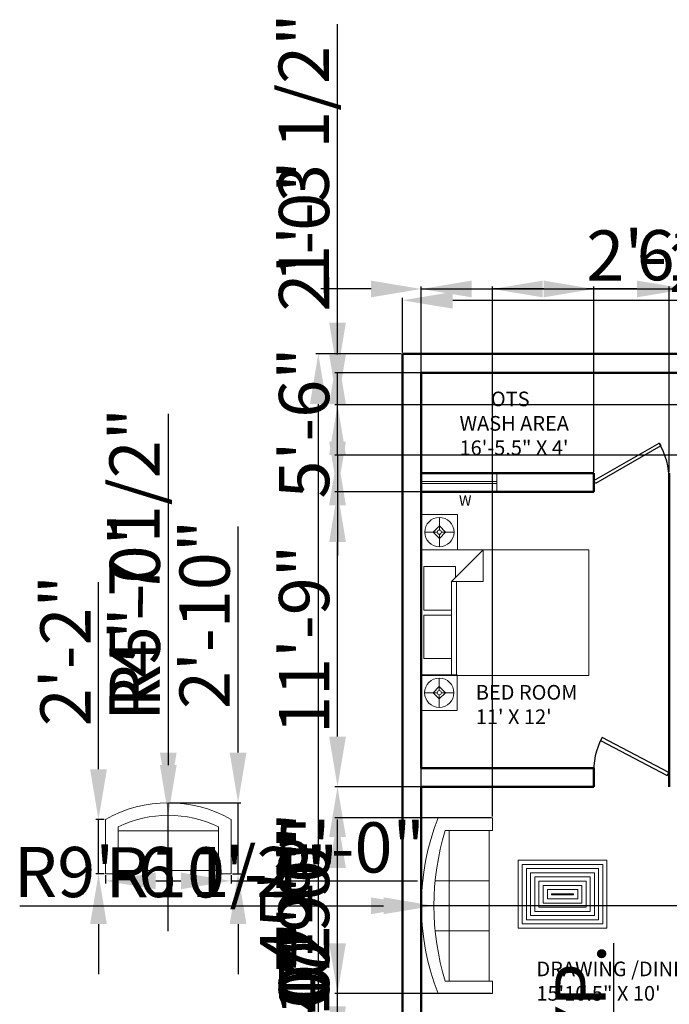
# Model space of a CAD drawing. Units: inches. Extents: x 1383 to 2465, y 1661 to 2415.
# Tile 2 of 4: x 1569 to 1880, y 1944 to 2415. Entities that reach past the tile are written whole.
import ezdxf

# ---------------------------------------------------------------- set-up
doc = ezdxf.new("R2010")
doc.units = ezdxf.units.IN
for name, color, linetype, lineweight in [('A-ANNO-DIMS', 2, 'Continuous', 18), ('A-ANNO-TEXT', 3, 'Continuous', 18), ('A-AREA-IDEN', 7, 'Continuous', 25), ('A-DOOR', 3, 'Continuous', 25), ('A-FURN', 8, 'Continuous', 18), ('A-GLAZ', 4, 'Continuous', 18), ('A-WALL', 7, 'Continuous', 50)]:
    doc.layers.add(name, color=color, linetype=linetype, lineweight=lineweight)
doc.styles.get("Standard").update_dxf_attribs({"font": 'arial.ttf'})
doc.dimstyles.new('ISO-25', dxfattribs={"dimtxt": 24, "dimasz": 24, "dimexe": 1.25, "dimexo": 0.625, "dimtad": 1, "dimdec": 0, "dimlunit": 3, "dimtxsty": 'Standard', "dimcen": 2.5, "dimadec": 0, "dimazin": 0, "dimtfac": 1, "dimtdec": 0, "dimtmove": 0, "dimatfit": 3, "dimfxl": 1, "dimarcsym": 0})

# ---------------------------------------------------------------- blocks, each defined once
blk = doc.blocks.new('*U4')
for p, q in [((0, 0), (0, -6)), ((-40, 0), (-40, -6))]:
    blk.add_line(p, q)
blk.add_lwpolyline([(0, 0), (-34.64, 20), (-35.52, 18.48), (-0.88, -1.52)], close=True)
blk.add_arc((0, 0), 40, 150, 180)
blk = doc.blocks.new('*U2')
for p, q in [((0, 0), (0, -6)), ((40, 0), (40, -6))]:
    blk.add_line(p, q)
blk.add_lwpolyline([(0, 0), (34.64, 20), (35.52, 18.48), (0.87, -1.52)], close=True)
blk.add_arc((0, 0), 40, 0, 30)
blk = doc.blocks.new('Bed - Queen')
for p, q in [((0, -80.00003), (0, 0)), ((0, 0), (59.99999, 0)), ((59.99999, 0), (59.99999, -80.00003)), ((7.99999, -1.2), (28.79998, -1.2)), ((7.99999, -14.4), (7.99999, -1.2)), ((28.79998, -1.2), (28.79998, -14.4)), ((31.19999, -1.2), (51.99999, -1.2)), ((31.19999, -14.4), (31.19999, -1.2)), ((51.99999, -1.2), (51.99999, -16.4)), ((0, -14.4), (44.8, -14.4)), ((44.8, -16.8), (0, -16.8)), ((59.99999, -29.6), (44.8, -14.4)), ((44.8, -14.4), (44.8, -29.6)), ((51.99999, -16.4), (46.79936, -16.4)), ((44.8, -29.6), (59.99999, -29.6)), ((59.99999, -80.00003), (0, -80.00003))]:
    blk.add_line(p, q)
blk = doc.blocks.new('Sofa - Roundback 7 ft.')
for p, q in [((-12.00002, -32.4421), (-12.00003, -6.5971)), ((11.99997, -32.4421), (11.99998, -6.5971)), ((-36.000027, -34), (-36.000027, -11.4696)), ((-35.999844, -13.3819), (35.9998, -13.3819)), ((35.99998, -34), (35.99998, -11.4696)), ((-36.000027, -32.4421), (35.99998, -32.4421))]:
    blk.add_line(p, q)
for points in [[(-36.000027, -34), (-42.000027, -34), (-42.000027, -8)], [(41.99998, -8), (41.99998, -34), (35.99998, -34)]]:
    blk.add_lwpolyline(points)
for centre, radius, start, end in [((0, -114.25), 114.25, 68.43141, 111.5686), ((-0.00001, -127.1968), 121.1968, 72.72033, 107.2797)]:
    blk.add_arc(centre, radius, start, end)
blk = doc.blocks.new('Sofa - Roundback Loveseat 5 ft.')
for p, q in [((0, -32.44198), (0, -5.99998)), ((-24, -33.99998), (-24, -11.46958)), ((-23.9998, -13.38178), (23.99986, -13.38178)), ((24.00004, -33.99998), (24.00004, -11.46958)), ((-24, -32.44198), (24.00004, -32.44198))]:
    blk.add_line(p, q)
for points in [[(-24, -33.99998), (-30, -33.99998), (-30, -7.99998)], [(30.00004, -7.99998), (30.00004, -33.99998), (24.00004, -33.99998)]]:
    blk.add_lwpolyline(points)
for centre, radius, start, end in [((0, -60.24998), 60.24998, 60.13715, 119.8628), ((0, -61.38438), 55.38444, 64.32083, 115.6792)]:
    blk.add_arc(centre, radius, start, end)
blk = doc.blocks.new('*D12')
at = {"layer": 'A-ANNO-DIMS', "color": 0, "lineweight": -2, "transparency": 16777216}
for p, q in [((1752.19, 2255.79), (1752.19, 2282.04)), ((1776.19, 2280.79), (2028.19, 2280.79)), ((2052.19, 2255.79), (2052.19, 2282.04))]:
    blk.add_line(p, q, dxfattribs=at)
at = {"layer": 'A-ANNO-DIMS', "color": 0, "transparency": 16777216}
for points in [[(1776.19, 2284.79), (1776.19, 2276.79), (1752.19, 2280.79)], [(2028.19, 2284.79), (2028.19, 2276.79), (2052.19, 2280.79)]]:
    blk.add_solid(points, dxfattribs=at)
at = {"layer": 'Defpoints', "color": 0, "transparency": 16777216}
for p in [(2052.19, 2280.79), (1752.19, 2255.16), (2052.19, 2255.16)]:
    blk.add_point(p, dxfattribs=at)
at = {"layer": 'A-ANNO-DIMS', "color": 0, "transparency": 16777216, "insert": (1902.19, 2293.67), "char_height": 24, "attachment_point": 5}
blk.add_mtext("25'", dxfattribs=at)
blk = doc.blocks.new('*D13')
at = {"layer": 'A-ANNO-DIMS', "color": 0, "lineweight": -2, "transparency": 16777216}
for p, q in [((1751.57, 2255.16), (1710.71, 2255.16)), ((1711.96, 2231.16), (1711.96, 1739.16)), ((1751.57, 1715.16), (1710.71, 1715.16))]:
    blk.add_line(p, q, dxfattribs=at)
at = {"layer": 'A-ANNO-DIMS', "color": 0, "transparency": 16777216}
for points in [[(1707.96, 2231.16), (1715.96, 2231.16), (1711.96, 2255.16)], [(1707.96, 1739.16), (1715.96, 1739.16), (1711.96, 1715.16)]]:
    blk.add_solid(points, dxfattribs=at)
at = {"layer": 'Defpoints', "color": 0, "transparency": 16777216}
for p in [(1752.19, 2255.16), (1711.96, 1715.16), (1752.19, 1715.16)]:
    blk.add_point(p, dxfattribs=at)
at = {"layer": 'A-ANNO-DIMS', "color": 0, "transparency": 16777216, "insert": (1699.13, 1985.16), "char_height": 24, "attachment_point": 5, "rotation": 90}
blk.add_mtext("45'", dxfattribs=at)
blk = doc.blocks.new('WIN-36IN')
for p, q in [((0, 36), (9, 36)), ((0, 0), (0, 36)), ((4, 0), (4, 36)), ((5, 36), (5, 0)), ((9, 36), (9, 0)), ((9, 0), (0, 0))]:
    blk.add_line(p, q)
blk = doc.blocks.new('Lamp - Table')
for p, q in [((0, 7), (0, 1)), ((-1, 0), (-7, 0)), ((0, 3), (-3, 0)), ((-3, 0), (0, -3)), ((3, 0), (0, 3)), ((0, -3), (3, 0)), ((1, 0), (7, 0)), ((0, -1), (0, -7))]:
    blk.add_line(p, q)
for radius in [7, 1]:
    blk.add_circle((0, 0), radius)
blk = doc.blocks.new('NIGHTSTAND-WITH-LAMP')
blk.add_lwpolyline([(0, 0), (17.23, 0), (17.23, 16.98), (0, 16.98)], close=True)
blk.add_blockref('Lamp - Table', (8.62, 8.49))
blk = doc.blocks.new('*D21')
at = {"layer": 'A-ANNO-DIMS', "color": 0, "lineweight": -2, "transparency": 16777216}
for p, q in [((1853.19, 1801.92), (1853.19, 1973.47)), ((1841.82, 1801.92), (1854.44, 1801.92)), ((1853.19, 1765.92), (1853.19, 1777.92)), ((1841.82, 1741.92), (1854.44, 1741.92))]:
    blk.add_line(p, q, dxfattribs=at)
at = {"layer": 'A-ANNO-DIMS', "color": 0, "transparency": 16777216}
for points in [[(1849.19, 1777.92), (1857.19, 1777.92), (1853.19, 1801.92)], [(1849.19, 1765.92), (1857.19, 1765.92), (1853.19, 1741.92)]]:
    blk.add_solid(points, dxfattribs=at)
at = {"layer": 'Defpoints', "color": 0, "transparency": 16777216}
for p in [(1841.19, 1801.92), (1853.19, 1801.92), (1841.19, 1741.92)]:
    blk.add_point(p, dxfattribs=at)
at = {"layer": 'A-ANNO-DIMS', "color": 0, "transparency": 16777216, "insert": (1840.32, 1899.7), "char_height": 24, "attachment_point": 5, "rotation": 90}
blk.add_mtext('5\'-0" TYP.', dxfattribs=at)
blk = doc.blocks.new('*D24')
at = {"layer": 'A-ANNO-DIMS', "color": 0, "lineweight": -2, "transparency": 16777216}
for p, q in [((1721.14, 1919.16), (1721.14, 2009.18)), ((1792.57, 1919.16), (1719.89, 1919.16)), ((1721.14, 1886.16), (1721.14, 1895.16)), ((1760.57, 1862.16), (1719.89, 1862.16))]:
    blk.add_line(p, q, dxfattribs=at)
at = {"layer": 'A-ANNO-DIMS', "color": 0, "transparency": 16777216}
for points in [[(1717.14, 1895.16), (1725.14, 1895.16), (1721.14, 1919.16)], [(1717.14, 1886.16), (1725.14, 1886.16), (1721.14, 1862.16)]]:
    blk.add_solid(points, dxfattribs=at)
at = {"layer": 'Defpoints', "color": 0, "transparency": 16777216}
for p in [(1721.14, 1919.16), (1793.19, 1919.16), (1761.19, 1862.16)]:
    blk.add_point(p, dxfattribs=at)
at = {"layer": 'A-ANNO-DIMS', "color": 0, "transparency": 16777216, "insert": (1708.26, 1976.17), "char_height": 24, "attachment_point": 5, "rotation": 90}
blk.add_mtext('4\'-9"', dxfattribs=at)
blk = doc.blocks.new('*D25')
at = {"layer": 'A-ANNO-DIMS', "color": 0, "lineweight": -2, "transparency": 16777216}
for p, q in [((1760.57, 2048.16), (1719.89, 2048.16)), ((1721.14, 1943.16), (1721.14, 2024.16)), ((1792.57, 1919.16), (1719.89, 1919.16))]:
    blk.add_line(p, q, dxfattribs=at)
at = {"layer": 'A-ANNO-DIMS', "color": 0, "transparency": 16777216}
for points in [[(1717.14, 2024.16), (1725.14, 2024.16), (1721.14, 2048.16)], [(1717.14, 1943.16), (1725.14, 1943.16), (1721.14, 1919.16)]]:
    blk.add_solid(points, dxfattribs=at)
at = {"layer": 'Defpoints', "color": 0, "transparency": 16777216}
for p in [(1721.14, 2048.16), (1761.19, 2048.16), (1793.19, 1919.16)]:
    blk.add_point(p, dxfattribs=at)
at = {"layer": 'A-ANNO-DIMS', "color": 0, "transparency": 16777216, "insert": (1708.26, 1983.66), "char_height": 24, "attachment_point": 5, "rotation": 90}
blk.add_mtext('10\'-9"', dxfattribs=at)
blk = doc.blocks.new('*D26')
at = {"layer": 'A-ANNO-DIMS', "color": 0, "lineweight": -2, "transparency": 16777216}
for p, q in [((1760.57, 2189.16), (1719.89, 2189.16)), ((1721.14, 2072.16), (1721.14, 2165.16)), ((1760.57, 2048.16), (1719.89, 2048.16))]:
    blk.add_line(p, q, dxfattribs=at)
at = {"layer": 'A-ANNO-DIMS', "color": 0, "transparency": 16777216}
for points in [[(1717.14, 2165.16), (1725.14, 2165.16), (1721.14, 2189.16)], [(1717.14, 2072.16), (1725.14, 2072.16), (1721.14, 2048.16)]]:
    blk.add_solid(points, dxfattribs=at)
at = {"layer": 'Defpoints', "color": 0, "transparency": 16777216}
for p in [(1721.14, 2189.16), (1761.19, 2189.16), (1761.19, 2048.16)]:
    blk.add_point(p, dxfattribs=at)
at = {"layer": 'A-ANNO-DIMS', "color": 0, "transparency": 16777216, "insert": (1708.26, 2118.66), "char_height": 24, "attachment_point": 5, "rotation": 90}
blk.add_mtext('11\'-9"', dxfattribs=at)
blk = doc.blocks.new('*D27')
at = {"layer": 'A-ANNO-DIMS', "color": 0, "lineweight": -2, "transparency": 16777216}
for p, q in [((1751.57, 2255.16), (1719.89, 2255.16)), ((1721.14, 2213.16), (1721.14, 2231.16)), ((1760.57, 2189.16), (1719.89, 2189.16))]:
    blk.add_line(p, q, dxfattribs=at)
at = {"layer": 'A-ANNO-DIMS', "color": 0, "transparency": 16777216}
for points in [[(1717.14, 2231.16), (1725.14, 2231.16), (1721.14, 2255.16)], [(1717.14, 2213.16), (1725.14, 2213.16), (1721.14, 2189.16)]]:
    blk.add_solid(points, dxfattribs=at)
at = {"layer": 'Defpoints', "color": 0, "transparency": 16777216}
for p in [(1721.14, 2255.16), (1752.19, 2255.16), (1761.19, 2189.16)]:
    blk.add_point(p, dxfattribs=at)
at = {"layer": 'A-ANNO-DIMS', "color": 0, "transparency": 16777216, "insert": (1708.26, 2222.16), "char_height": 24, "attachment_point": 5, "rotation": 90}
blk.add_mtext('5\'-6"', dxfattribs=at)
blk = doc.blocks.new('*D28')
at = {"layer": 'A-ANNO-DIMS', "color": 0, "lineweight": -2, "transparency": 16777216}
for p, q in [((1606.91, 2056.55), (1606.91, 2146.01)), ((1609.63, 2032.55), (1605.66, 2032.55)), ((1606.91, 2006.55), (1606.91, 2032.55)), ((1609.63, 2006.55), (1605.66, 2006.55)), ((1606.91, 1982.55), (1606.91, 1958.55))]:
    blk.add_line(p, q, dxfattribs=at)
at = {"layer": 'A-ANNO-DIMS', "color": 0, "transparency": 16777216}
for points in [[(1602.91, 2056.55), (1610.91, 2056.55), (1606.91, 2032.55)], [(1602.91, 1982.55), (1610.91, 1982.55), (1606.91, 2006.55)]]:
    blk.add_solid(points, dxfattribs=at)
at = {"layer": 'Defpoints', "color": 0, "transparency": 16777216}
for p in [(1606.91, 2032.55), (1610.26, 2032.55), (1610.26, 2006.55)]:
    blk.add_point(p, dxfattribs=at)
at = {"layer": 'A-ANNO-DIMS', "color": 0, "transparency": 16777216, "insert": (1594.23, 2113.28), "char_height": 24, "attachment_point": 5, "rotation": 90}
blk.add_mtext('2\'-2"', dxfattribs=at)
blk = doc.blocks.new('*D29')
at = {"layer": 'A-ANNO-DIMS', "color": 0, "lineweight": -2, "transparency": 16777216}
for p, q in [((1610.26, 2005.92), (1610.26, 2001.95)), ((1670.26, 2005.92), (1670.26, 2001.95)), ((1634.26, 2003.2), (1646.26, 2003.2)), ((1670.26, 2003.2), (1759.31, 2003.2))]:
    blk.add_line(p, q, dxfattribs=at)
at = {"layer": 'A-ANNO-DIMS', "color": 0, "transparency": 16777216}
for points in [[(1634.26, 2007.2), (1634.26, 1999.2), (1610.26, 2003.2)], [(1646.26, 2007.2), (1646.26, 1999.2), (1670.26, 2003.2)]]:
    blk.add_solid(points, dxfattribs=at)
at = {"layer": 'Defpoints', "color": 0, "transparency": 16777216}
for p in [(1610.26, 2006.55), (1670.26, 2006.55), (1670.26, 2003.2)]:
    blk.add_point(p, dxfattribs=at)
at = {"layer": 'A-ANNO-DIMS', "color": 0, "transparency": 16777216, "insert": (1726.78, 2016.08), "char_height": 24, "attachment_point": 5}
blk.add_mtext('5\'-0"', dxfattribs=at)
blk = doc.blocks.new('*D30')
at = {"layer": 'A-ANNO-DIMS', "color": 0, "lineweight": -2, "transparency": 16777216}
for p, q in [((1673.61, 2064.55), (1673.61, 2172.65)), ((1640.88, 2040.55), (1674.86, 2040.55)), ((1673.61, 2006.55), (1673.61, 2040.55)), ((1670.88, 2006.55), (1674.86, 2006.55)), ((1673.61, 1982.55), (1673.61, 1958.55))]:
    blk.add_line(p, q, dxfattribs=at)
at = {"layer": 'A-ANNO-DIMS', "color": 0, "transparency": 16777216}
for points in [[(1669.61, 2064.55), (1677.61, 2064.55), (1673.61, 2040.55)], [(1669.61, 1982.55), (1677.61, 1982.55), (1673.61, 2006.55)]]:
    blk.add_solid(points, dxfattribs=at)
at = {"layer": 'Defpoints', "color": 0, "transparency": 16777216}
for p in [(1640.26, 2040.55), (1673.61, 2040.55), (1670.26, 2006.55)]:
    blk.add_point(p, dxfattribs=at)
at = {"layer": 'A-ANNO-DIMS', "color": 0, "transparency": 16777216, "insert": (1660.73, 2130.6), "char_height": 24, "attachment_point": 5, "rotation": 90}
blk.add_mtext('2\'-10"', dxfattribs=at)
blk = doc.blocks.new('*D34')
at = {"layer": 'A-ANNO-DIMS', "color": 0, "lineweight": -2, "transparency": 16777216}
for p, q in [((1721.14, 2254.82), (1721.14, 2344.28)), ((2042.57, 2230.82), (1719.89, 2230.82)), ((1721.14, 2206.82), (1721.14, 2230.82)), ((2042.57, 2206.82), (1719.89, 2206.82)), ((1721.14, 2182.82), (1721.14, 2158.82))]:
    blk.add_line(p, q, dxfattribs=at)
at = {"layer": 'A-ANNO-DIMS', "color": 0, "transparency": 16777216}
for points in [[(1717.14, 2254.82), (1725.14, 2254.82), (1721.14, 2230.82)], [(1717.14, 2182.82), (1725.14, 2182.82), (1721.14, 2206.82)]]:
    blk.add_solid(points, dxfattribs=at)
at = {"layer": 'Defpoints', "color": 0, "transparency": 16777216}
for p in [(1721.14, 2230.82), (2043.19, 2230.82), (2043.19, 2206.82)]:
    blk.add_point(p, dxfattribs=at)
at = {"layer": 'A-ANNO-DIMS', "color": 0, "transparency": 16777216, "insert": (1708.26, 2311.55), "char_height": 24, "attachment_point": 5, "rotation": 90}
blk.add_mtext('2\'-0"', dxfattribs=at)
blk = doc.blocks.new('*D35')
at = {"layer": 'A-ANNO-DIMS', "color": 0, "lineweight": -2, "transparency": 16777216}
for p, q in [((1721.14, 2270.16), (1721.14, 2412.87)), ((2042.57, 2246.16), (1719.89, 2246.16)), ((1721.14, 2230.82), (1721.14, 2246.16)), ((2042.57, 2230.82), (1719.89, 2230.82)), ((1721.14, 2206.82), (1721.14, 2182.82))]:
    blk.add_line(p, q, dxfattribs=at)
at = {"layer": 'A-ANNO-DIMS', "color": 0, "transparency": 16777216}
for points in [[(1717.14, 2270.16), (1725.14, 2270.16), (1721.14, 2246.16)], [(1717.14, 2206.82), (1725.14, 2206.82), (1721.14, 2230.82)]]:
    blk.add_solid(points, dxfattribs=at)
at = {"layer": 'Defpoints', "color": 0, "transparency": 16777216}
for p in [(1721.14, 2246.16), (2043.19, 2246.16), (2043.19, 2230.82)]:
    blk.add_point(p, dxfattribs=at)
at = {"layer": 'A-ANNO-DIMS', "color": 0, "transparency": 16777216, "insert": (1708.1, 2353.52), "char_height": 24, "attachment_point": 5, "rotation": 90}
blk.add_mtext('1\'-3 1/2"', dxfattribs=at)
blk = doc.blocks.new('*D38')
at = {"layer": 'A-ANNO-DIMS', "color": 0, "lineweight": -2, "transparency": 16777216}
for p, q in [((1761.19, 2198.79), (1761.19, 2287.46)), ((1785.19, 2286.21), (1819.69, 2286.21)), ((1843.69, 2198.79), (1843.69, 2287.46)), ((1843.69, 2286.21), (2007.44, 2286.21))]:
    blk.add_line(p, q, dxfattribs=at)
at = {"layer": 'A-ANNO-DIMS', "color": 0, "transparency": 16777216}
for points in [[(1785.19, 2290.21), (1785.19, 2282.21), (1761.19, 2286.21)], [(1819.69, 2290.21), (1819.69, 2282.21), (1843.69, 2286.21)]]:
    blk.add_solid(points, dxfattribs=at)
at = {"layer": 'Defpoints', "color": 0, "transparency": 16777216}
for p in [(1843.69, 2286.21), (1761.19, 2198.16), (1843.69, 2198.16)]:
    blk.add_point(p, dxfattribs=at)
at = {"layer": 'A-ANNO-DIMS', "color": 0, "transparency": 16777216, "insert": (1937.57, 2299.25), "char_height": 24, "attachment_point": 5}
blk.add_mtext('6\'-10 1/2"', dxfattribs=at)
blk = doc.blocks.new('*D39')
at = {"layer": 'A-ANNO-DIMS', "color": 0, "lineweight": -2, "transparency": 16777216}
for p, q in [((1819.69, 2286.21), (1795.69, 2286.21)), ((1843.69, 2198.79), (1843.69, 2287.46)), ((1843.69, 2286.21), (1879.69, 2286.21)), ((1879.69, 2198.79), (1879.69, 2287.46)), ((1903.69, 2286.21), (1992.73, 2286.21))]:
    blk.add_line(p, q, dxfattribs=at)
at = {"layer": 'A-ANNO-DIMS', "color": 0, "transparency": 16777216}
for points in [[(1819.69, 2290.21), (1819.69, 2282.21), (1843.69, 2286.21)], [(1903.69, 2290.21), (1903.69, 2282.21), (1879.69, 2286.21)]]:
    blk.add_solid(points, dxfattribs=at)
at = {"layer": 'Defpoints', "color": 0, "transparency": 16777216}
for p in [(1879.69, 2286.21), (1843.69, 2198.16), (1879.69, 2198.16)]:
    blk.add_point(p, dxfattribs=at)
at = {"layer": 'A-ANNO-DIMS', "color": 0, "transparency": 16777216, "insert": (1960.21, 2299.1), "char_height": 24, "attachment_point": 5}
blk.add_mtext('3\'-0"', dxfattribs=at)
blk = doc.blocks.new('*D41')
at = {"layer": 'A-ANNO-DIMS', "color": 0, "lineweight": -2, "transparency": 16777216}
for p, q in [((1721.14, 1943.16), (1721.14, 2032.62)), ((1792.57, 1919.16), (1719.89, 1919.16)), ((1721.14, 1895.16), (1721.14, 1919.16)), ((1792.57, 1895.16), (1719.89, 1895.16)), ((1721.14, 1871.16), (1721.14, 1847.16))]:
    blk.add_line(p, q, dxfattribs=at)
at = {"layer": 'A-ANNO-DIMS', "color": 0, "transparency": 16777216}
for points in [[(1717.14, 1943.16), (1725.14, 1943.16), (1721.14, 1919.16)], [(1717.14, 1871.16), (1725.14, 1871.16), (1721.14, 1895.16)]]:
    blk.add_solid(points, dxfattribs=at)
at = {"layer": 'Defpoints', "color": 0, "transparency": 16777216}
for p in [(1721.14, 1919.16), (1793.19, 1919.16), (1793.19, 1895.16)]:
    blk.add_point(p, dxfattribs=at)
at = {"layer": 'A-ANNO-DIMS', "color": 0, "transparency": 16777216, "insert": (1708.26, 1999.89), "char_height": 24, "attachment_point": 5, "rotation": 90}
blk.add_mtext('2\'-0"', dxfattribs=at)
blk = doc.blocks.new('*D47')
at = {"layer": 'A-ANNO-DIMS', "color": 0, "lineweight": -2, "transparency": 16777216}
for p, q in [((1721.14, 1883.16), (1721.14, 1972.21)), ((1946.57, 1883.16), (1719.89, 1883.16)), ((1721.14, 1847.16), (1721.14, 1859.16)), ((1946.57, 1823.16), (1719.89, 1823.16))]:
    blk.add_line(p, q, dxfattribs=at)
at = {"layer": 'A-ANNO-DIMS', "color": 0, "transparency": 16777216}
for points in [[(1717.14, 1859.16), (1725.14, 1859.16), (1721.14, 1883.16)], [(1717.14, 1847.16), (1725.14, 1847.16), (1721.14, 1823.16)]]:
    blk.add_solid(points, dxfattribs=at)
at = {"layer": 'Defpoints', "color": 0, "transparency": 16777216}
for p in [(1721.14, 1883.16), (1947.19, 1883.16), (1947.19, 1823.16)]:
    blk.add_point(p, dxfattribs=at)
at = {"layer": 'A-ANNO-DIMS', "color": 0, "transparency": 16777216, "insert": (1708.26, 1939.69), "char_height": 24, "attachment_point": 5, "rotation": 90}
blk.add_mtext('5\'-0"', dxfattribs=at)
blk = doc.blocks.new('*D48')
at = {"layer": 'A-ANNO-DIMS', "color": 0, "lineweight": -2, "transparency": 16777216}
for p, q in [((1794.57, 2033.3), (1719.89, 2033.3)), ((1721.14, 1973.3), (1721.14, 2009.3)), ((1794.57, 1949.3), (1719.89, 1949.3))]:
    blk.add_line(p, q, dxfattribs=at)
at = {"layer": 'A-ANNO-DIMS', "color": 0, "transparency": 16777216}
for points in [[(1717.14, 2009.3), (1725.14, 2009.3), (1721.14, 2033.3)], [(1717.14, 1973.3), (1725.14, 1973.3), (1721.14, 1949.3)]]:
    blk.add_solid(points, dxfattribs=at)
at = {"layer": 'Defpoints', "color": 0, "transparency": 16777216}
for p in [(1721.14, 2033.3), (1795.19, 2033.3), (1795.19, 1949.3)]:
    blk.add_point(p, dxfattribs=at)
at = {"layer": 'A-ANNO-DIMS', "color": 0, "transparency": 16777216, "insert": (1708.26, 1991.3), "char_height": 24, "attachment_point": 5, "rotation": 90}
blk.add_mtext('7\'-0"', dxfattribs=at)
blk = doc.blocks.new('*D49')
at = {"layer": 'A-ANNO-DIMS', "color": 0, "lineweight": -2, "transparency": 16777216}
for p, q in [((1737.19, 2286.21), (1713.19, 2286.21)), ((1761.19, 1991.92), (1761.19, 2287.46)), ((1761.19, 2286.21), (1795.19, 2286.21)), ((1795.19, 2033.92), (1795.19, 2287.46)), ((1819.19, 2286.21), (1927.3, 2286.21))]:
    blk.add_line(p, q, dxfattribs=at)
at = {"layer": 'A-ANNO-DIMS', "color": 0, "transparency": 16777216}
for points in [[(1737.19, 2290.21), (1737.19, 2282.21), (1761.19, 2286.21)], [(1819.19, 2290.21), (1819.19, 2282.21), (1795.19, 2286.21)]]:
    blk.add_solid(points, dxfattribs=at)
at = {"layer": 'Defpoints', "color": 0, "transparency": 16777216}
for p in [(1795.19, 2286.21), (1795.19, 2033.3), (1761.19, 1991.3)]:
    blk.add_point(p, dxfattribs=at)
at = {"layer": 'A-ANNO-DIMS', "color": 0, "transparency": 16777216, "insert": (1885.25, 2299.09), "char_height": 24, "attachment_point": 5}
blk.add_mtext('2\'-10"', dxfattribs=at)
blk = doc.blocks.new('*D50')
at = {"layer": 'A-ANNO-DIMS', "color": 0, "lineweight": -2, "transparency": 16777216}
for p, q in [((1864.19, 2286.21), (1840.19, 2286.21)), ((1888.19, 1919.79), (1888.19, 2287.46)), ((1888.19, 2286.21), (1924.19, 2286.21)), ((1924.19, 1919.79), (1924.19, 2287.46)), ((1948.19, 2286.21), (2037.23, 2286.21))]:
    blk.add_line(p, q, dxfattribs=at)
at = {"layer": 'A-ANNO-DIMS', "color": 0, "transparency": 16777216}
for points in [[(1864.19, 2290.21), (1864.19, 2282.21), (1888.19, 2286.21)], [(1948.19, 2290.21), (1948.19, 2282.21), (1924.19, 2286.21)]]:
    blk.add_solid(points, dxfattribs=at)
at = {"layer": 'Defpoints', "color": 0, "transparency": 16777216}
for p in [(1924.19, 2286.21), (1888.19, 1919.16), (1924.19, 1919.16)]:
    blk.add_point(p, dxfattribs=at)
at = {"layer": 'A-ANNO-DIMS', "color": 0, "transparency": 16777216, "insert": (2004.71, 2299.1), "char_height": 24, "attachment_point": 5}
blk.add_mtext('3\'-0"', dxfattribs=at)
blk = doc.blocks.new('*D53')
at = {"layer": 'A-ANNO-DIMS', "color": 0, "lineweight": -2, "transparency": 16777216}
for p, q in [((1721.14, 1886.16), (1721.14, 1975.19)), ((1887.57, 1862.16), (1719.89, 1862.16)), ((1721.14, 1826.16), (1721.14, 1862.16)), ((1887.57, 1826.16), (1719.89, 1826.16)), ((1721.14, 1802.16), (1721.14, 1778.16))]:
    blk.add_line(p, q, dxfattribs=at)
at = {"layer": 'A-ANNO-DIMS', "color": 0, "transparency": 16777216}
for points in [[(1717.14, 1886.16), (1725.14, 1886.16), (1721.14, 1862.16)], [(1717.14, 1802.16), (1725.14, 1802.16), (1721.14, 1826.16)]]:
    blk.add_solid(points, dxfattribs=at)
at = {"layer": 'Defpoints', "color": 0, "transparency": 16777216}
for p in [(1721.14, 1862.16), (1888.19, 1862.16), (1888.19, 1826.16)]:
    blk.add_point(p, dxfattribs=at)
at = {"layer": 'A-ANNO-DIMS', "color": 0, "transparency": 16777216, "insert": (1708.26, 1942.68), "char_height": 24, "attachment_point": 5, "rotation": 90}
blk.add_mtext('3\'-0"', dxfattribs=at)
blk = doc.blocks.new('*D54')
at = {"layer": 'A-ANNO-DIMS', "color": 0, "lineweight": -2, "transparency": 16777216}
for p, q in [((1612.53, 1991.3), (1743.19, 1991.3)), ((1888.39, 1991.3), (1767.19, 1991.3))]:
    blk.add_line(p, q, dxfattribs=at)
at = {"layer": 'A-ANNO-DIMS', "color": 0, "transparency": 16777216}
blk.add_solid([(1743.19, 1995.3), (1743.19, 1987.3), (1767.19, 1991.3)], dxfattribs=at)
at = {"layer": 'Defpoints', "color": 0, "transparency": 16777216}
for p in [(1767.19, 1991.3), (1888.39, 1991.3)]:
    blk.add_point(p, dxfattribs=at)
at = {"layer": 'A-ANNO-DIMS', "color": 0, "transparency": 16777216, "insert": (1665.86, 2004.17), "char_height": 24, "attachment_point": 5, "rotation": 359.9999}
blk.add_mtext('R10\'-1"', dxfattribs=at)
blk = doc.blocks.new('*D55')
at = {"layer": 'A-ANNO-DIMS', "color": 0, "lineweight": -2, "transparency": 16777216}
for p, q in [((1569.25, 1991.3), (1737.19, 1991.3)), ((1875.44, 1991.3), (1761.19, 1991.3))]:
    blk.add_line(p, q, dxfattribs=at)
at = {"layer": 'A-ANNO-DIMS', "color": 0, "transparency": 16777216}
blk.add_solid([(1737.19, 1995.3), (1737.19, 1987.3), (1761.19, 1991.3)], dxfattribs=at)
at = {"layer": 'Defpoints', "color": 0, "transparency": 16777216}
for p in [(1761.19, 1991.3), (1875.44, 1991.3)]:
    blk.add_point(p, dxfattribs=at)
at = {"layer": 'A-ANNO-DIMS', "color": 0, "transparency": 16777216, "insert": (1641.22, 2004.33), "char_height": 24, "attachment_point": 5, "rotation": 359.9999}
blk.add_mtext('R9\'-6 1/2"', dxfattribs=at)
blk = doc.blocks.new('*D56')
at = {"layer": 'A-ANNO-DIMS', "color": 0, "lineweight": -2, "transparency": 16777216}
for p, q in [((1640.26, 2176.57), (1640.26, 2064.55)), ((1640.26, 1980.3), (1640.26, 2040.55))]:
    blk.add_line(p, q, dxfattribs=at)
at = {"layer": 'A-ANNO-DIMS', "color": 0, "transparency": 16777216}
blk.add_solid([(1636.26, 2064.55), (1644.26, 2064.55), (1640.26, 2040.55)], dxfattribs=at)
at = {"layer": 'Defpoints', "color": 0, "transparency": 16777216}
for p in [(1640.26, 2040.55), (1640.26, 1980.3)]:
    blk.add_point(p, dxfattribs=at)
at = {"layer": 'A-ANNO-DIMS', "color": 0, "transparency": 16777216, "insert": (1627.38, 2132.56), "char_height": 24, "attachment_point": 5, "rotation": 89.9987}
blk.add_mtext('R5\'-0"', dxfattribs=at)
blk = doc.blocks.new('*D57')
at = {"layer": 'A-ANNO-DIMS', "color": 0, "lineweight": -2, "transparency": 16777216}
for p, q in [((1640.26, 2226.49), (1640.26, 2058.55)), ((1640.26, 1979.16), (1640.26, 2034.55))]:
    blk.add_line(p, q, dxfattribs=at)
at = {"layer": 'A-ANNO-DIMS', "color": 0, "transparency": 16777216}
blk.add_solid([(1636.26, 2058.55), (1644.26, 2058.55), (1640.26, 2034.55)], dxfattribs=at)
at = {"layer": 'Defpoints', "color": 0, "transparency": 16777216}
for p in [(1640.26, 2034.55), (1640.26, 1979.16)]:
    blk.add_point(p, dxfattribs=at)
at = {"layer": 'A-ANNO-DIMS', "color": 0, "transparency": 16777216, "insert": (1627.23, 2154.52), "char_height": 24, "attachment_point": 5, "rotation": 89.9986}
blk.add_mtext('R4\'-7 1/2"', dxfattribs=at)

msp = doc.modelspace()

# ---------------------------------------------------------------- linework, layer by layer
at = {"layer": 'A-FURN'}
for points in [[(1807.41, 2013.07), (1849.91, 2013.07), (1849.91, 1980.59), (1807.41, 1980.59)], [(1809.41, 2011.07), (1847.91, 2011.07), (1847.91, 1982.59), (1809.41, 1982.59)], [(1811.41, 2009.07), (1845.91, 2009.07), (1845.91, 1984.59), (1811.41, 1984.59)], [(1813.41, 2007.07), (1843.91, 2007.07), (1843.91, 1986.59), (1813.41, 1986.59)], [(1815.41, 2005.07), (1841.91, 2005.07), (1841.91, 1988.59), (1815.41, 1988.59)], [(1817.41, 2003.07), (1839.91, 2003.07), (1839.91, 1990.59), (1817.41, 1990.59)], [(1819.41, 2001.07), (1837.91, 2001.07), (1837.91, 1992.59), (1819.41, 1992.59)], [(1821.41, 1999.07), (1835.91, 1999.07), (1835.91, 1994.59), (1821.41, 1994.59)], [(1823.41, 1997.07), (1833.91, 1997.07), (1833.91, 1996.59), (1823.41, 1996.59)]]:
    msp.add_lwpolyline(points, close=True, dxfattribs=at)
at = {"layer": 'A-WALL'}
for p, q in [((1761.19, 2246.16), (2043.19, 2246.16)), ((1761.19, 2057.16), (1761.19, 2246.16)), ((1761.19, 2198.16), (1843.69, 2198.16)), ((1843.69, 2189.16), (1843.69, 2198.16)), ((1879.69, 2198.16), (1879.69, 2048.16)), ((1879.69, 2189.16), (1879.69, 2198.16)), ((1761.19, 2189.16), (1843.69, 2189.16)), ((1761.19, 2057.16), (1843.69, 2057.16)), ((1843.69, 2057.16), (1843.69, 2048.16)), ((1879.69, 2057.16), (1879.69, 2048.16)), ((1761.19, 2048.16), (1843.69, 2048.16)), ((1761.19, 1871.16), (1761.19, 2048.16))]:
    msp.add_line(p, q, dxfattribs=at)
msp.add_lwpolyline([(1752.19, 2255.16), (2052.19, 2255.16), (2052.19, 1715.16), (1752.19, 1715.16)], close=True, dxfattribs=at)

# ---------------------------------------------------------------- block references
at = {"layer": 'A-DOOR', "xscale": 0.9000000000000058, "yscale": 0.9000000000000058, "zscale": 0.9000000000000058}
msp.add_blockref('*U2', (1843.69, 2194.56), dxfattribs=at)
at = {"layer": 'A-DOOR', "xscale": 0.9006830181943749, "yscale": 0.9006830181943749, "zscale": 0.9006830181943749, "rotation": 2.231491455052545}
msp.add_blockref('*U4', (1879.48, 2054.97), dxfattribs=at)
at = {"layer": 'A-FURN'}
for name, p in [('NIGHTSTAND-WITH-LAMP', (1761.19, 2161.47)), ('NIGHTSTAND-WITH-LAMP', (1761.16, 2084.68)), ('Sofa - Roundback Loveseat 5 ft.', (1640.26, 2040.55))]:
    msp.add_blockref(name, p, dxfattribs=at)
at = {"layer": 'A-FURN', "rotation": 90}
for name, p in [('Bed - Queen', (1761.19, 2101.47)), ('Sofa - Roundback 7 ft.', (1761.19, 1991.3))]:
    msp.add_blockref(name, p, dxfattribs=at)
at = {"layer": 'A-GLAZ', "rotation": 269.9999999999983}
msp.add_blockref('WIN-36IN', (1761.28, 2198.16), dxfattribs=at)

# ---------------------------------------------------------------- texts
at = {"layer": 'A-ANNO-TEXT', "insert": (1779.18, 2187.57), "char_height": 5, "attachment_point": 1}
msp.add_mtext_dynamic_manual_height_columns('{\\fArial|b1|i0|c0|p34;W}', width=53.5912, gutter_width=12.5, heights=[38.86], dxfattribs=at)
at = {"layer": 'A-AREA-IDEN', "char_height": 7, "attachment_point": 1}
for s, width, heights, insert in [('{\\fArial|b1|i0|c0|p34;       OTS\\PWASH AREA\\P16\'-5.5" X 4\'}', 98.0388, [34.41], (1779.45, 2237.13)), ("{\\fArial|b1|i0|c0|p34;BED ROOM\\P11' X 12'}", 53.5912, [38.86], (1787.22, 2096.86)), ('{\\fArial|b1|i0|c0|p34;DRAWING /DINING\\P15\'10.5" X 10\'}', 95.0663, [44.26], (1816.2, 1964.61))]:
    msp.add_mtext_dynamic_manual_height_columns(s, width=width, gutter_width=12.5, heights=heights, dxfattribs=dict(at, insert=insert))

# ---------------------------------------------------------------- dimensions: what is measured, and where the dimension line sits
at = {"layer": 'A-ANNO-DIMS'}
for base, p1, p2, override, picture, middle in [((1721.14, 2246.16), (2043.19, 2230.82), (2043.19, 2246.16), {"dimdec": 1, "dimlfac": 1, "dimrnd": 0, "dimzin": 1, "dimdsep": 46, "dimlunit": 4, "dimfrac": 2}, '*D35', (1708.1, 2353.52)), ((1721.14, 2230.82), (2043.19, 2206.82), (2043.19, 2230.82), {"dimdec": 1, "dimlfac": 1, "dimrnd": 0, "dimzin": 1, "dimdsep": 46, "dimlunit": 4, "dimfrac": 2}, '*D34', (1708.26, 2311.55)), ((1711.96, 1715.16), (1752.19, 2255.16), (1752.19, 1715.16), {"dimclrd": 0, "dimclre": 0, "dimclrt": 0}, '*D13', (1699.13, 1985.16)), ((1721.14, 2255.16), (1761.19, 2189.16), (1752.19, 2255.16), {"dimdec": 1, "dimlfac": 1, "dimrnd": 0, "dimzin": 1, "dimdsep": 46, "dimlunit": 4, "dimfrac": 2}, '*D27', (1708.26, 2222.16)), ((1721.14, 2189.16), (1761.19, 2048.16), (1761.19, 2189.16), {"dimdec": 1, "dimlfac": 1, "dimrnd": 0, "dimzin": 1, "dimdsep": 46, "dimlunit": 4, "dimfrac": 2}, '*D26', (1708.26, 2118.66)), ((1673.61, 2040.55), (1670.26, 2006.55), (1640.26, 2040.55), {"dimdec": 1, "dimlfac": 1, "dimrnd": 0, "dimzin": 1, "dimdsep": 46, "dimlunit": 4, "dimfrac": 2}, '*D30', (1660.73, 2130.6)), ((1606.91, 2032.55), (1610.26, 2006.55), (1610.26, 2032.55), {"dimdec": 1, "dimlfac": 1, "dimrnd": 0, "dimzin": 1, "dimdsep": 46, "dimlunit": 4, "dimfrac": 2}, '*D28', (1594.23, 2113.28)), ((1721.14, 2048.16), (1793.19, 1919.16), (1761.19, 2048.16), {"dimdec": 1, "dimlfac": 1, "dimrnd": 0, "dimzin": 1, "dimdsep": 46, "dimlunit": 4, "dimfrac": 2}, '*D25', (1708.26, 1983.66)), ((1721.14, 1919.16), (1793.19, 1895.16), (1793.19, 1919.16), {"dimdec": 1, "dimlfac": 1, "dimrnd": 0, "dimzin": 1, "dimdsep": 46, "dimlunit": 4, "dimfrac": 2}, '*D41', (1708.26, 1999.89)), ((1721.14, 2033.3), (1795.19, 1949.3), (1795.19, 2033.3), {"dimdec": 1, "dimlfac": 1, "dimrnd": 0, "dimzin": 1, "dimdsep": 46, "dimlunit": 4, "dimfrac": 2}, '*D48', (1708.26, 1991.3)), ((1721.14, 1919.16), (1761.19, 1862.16), (1793.19, 1919.16), {"dimdec": 1, "dimlfac": 1, "dimrnd": 0, "dimzin": 1, "dimdsep": 46, "dimlunit": 4, "dimfrac": 2}, '*D24', (1708.26, 1976.17)), ((1721.14, 1862.16), (1888.19, 1826.16), (1888.19, 1862.16), {"dimdec": 1, "dimlfac": 1, "dimrnd": 0, "dimzin": 1, "dimdsep": 46, "dimlunit": 4, "dimfrac": 2}, '*D53', (1708.26, 1942.68)), ((1721.14, 1883.16), (1947.19, 1823.16), (1947.19, 1883.16), {"dimdec": 1, "dimlfac": 1, "dimrnd": 0, "dimzin": 1, "dimdsep": 46, "dimlunit": 4, "dimfrac": 2}, '*D47', (1708.26, 1939.69))]:
    dim = msp.add_linear_dim(base=base, p1=p1, p2=p2, angle=90, dimstyle='ISO-25', override=override, dxfattribs=at)
    dim.commit()
    dim.dimension.update_dxf_attribs({"geometry": picture, "text_midpoint": middle})
for base, p1, p2, override, picture, middle in [((1843.69, 2286.21), (1761.19, 2198.16), (1843.69, 2198.16), {"dimdec": 1, "dimlfac": 1, "dimrnd": 0, "dimzin": 1, "dimdsep": 46, "dimlunit": 4, "dimfrac": 2}, '*D38', (1937.57, 2299.25)), ((1795.19, 2286.21), (1761.19, 1991.3), (1795.19, 2033.3), {"dimdec": 1, "dimlfac": 1, "dimrnd": 0, "dimzin": 1, "dimdsep": 46, "dimlunit": 4, "dimfrac": 2}, '*D49', (1885.25, 2299.09)), ((1879.69, 2286.21), (1843.69, 2198.16), (1879.69, 2198.16), {"dimdec": 1, "dimlfac": 1, "dimrnd": 0, "dimzin": 1, "dimdsep": 46, "dimlunit": 4, "dimfrac": 2}, '*D39', (1960.21, 2299.1)), ((1924.19, 2286.21), (1888.19, 1919.16), (1924.19, 1919.16), {"dimdec": 1, "dimlfac": 1, "dimrnd": 0, "dimzin": 1, "dimdsep": 46, "dimlunit": 4, "dimfrac": 2}, '*D50', (2004.71, 2299.1)), ((2052.19, 2280.79), (1752.19, 2255.16), (2052.19, 2255.16), {"dimclrd": 0, "dimclre": 0, "dimclrt": 0}, '*D12', (1902.19, 2293.67)), ((1670.26, 2003.2), (1610.26, 2006.55), (1670.26, 2006.55), {"dimdec": 1, "dimlfac": 1, "dimrnd": 0, "dimzin": 1, "dimdsep": 46, "dimlunit": 4, "dimfrac": 2}, '*D29', (1726.78, 2016.08))]:
    dim = msp.add_linear_dim(base=base, p1=p1, p2=p2, dimstyle='ISO-25', override=override, dxfattribs=at)
    dim.commit()
    dim.dimension.update_dxf_attribs({"geometry": picture, "text_midpoint": middle})
for center, mpoint, picture, middle in [((1640.26, 1979.16), (1640.26, 2034.55), '*D57', (1627.23, 2154.52)), ((1640.2587, 1980.2988), (1640.26, 2040.5487), '*D56', (1627.3833, 2132.5574)), ((1875.443743, 1991.295849), (1761.193743, 1991.296), '*D55', (1641.22360334, 2004.3304355)), ((1888.39, 1991.3), (1767.19, 1991.3), '*D54', (1665.86, 2004.17))]:
    dim = msp.add_radius_dim(center=center, mpoint=mpoint, dimstyle='ISO-25', override={"dimdec": 1, "dimlfac": 1, "dimrnd": 0, "dimzin": 1, "dimdsep": 46, "dimlunit": 4, "dimfrac": 2}, dxfattribs=at)
    dim.commit()
    dim.dimension.update_dxf_attribs({"geometry": picture, "text_midpoint": middle})
dim = msp.add_linear_dim(base=(1853.19, 1801.92), p1=(1841.19, 1741.92), p2=(1841.19, 1801.92), angle=90, text='<> TYP.', dimstyle='ISO-25', override={"dimdec": 1, "dimlfac": 1, "dimrnd": 0, "dimzin": 1, "dimdsep": 46, "dimlunit": 4, "dimfrac": 2}, dxfattribs=at)
dim.commit()
dim.dimension.update_dxf_attribs({"geometry": '*D21', "text_midpoint": (1840.32, 1899.7)})

doc.saveas('drawing.dxf')
